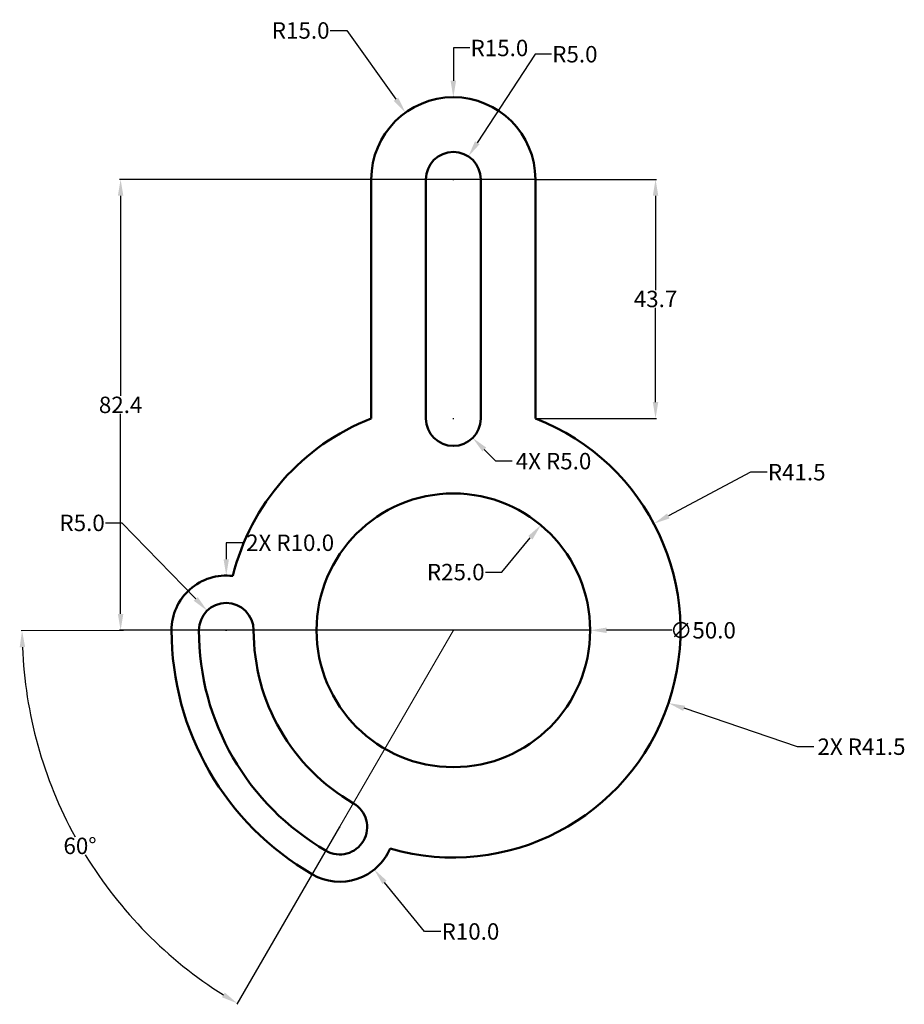
# Model space of a CAD drawing. Units: millimetres. Extents: x 927 to 1089, y 1498 to 1678.
import ezdxf

# ---------------------------------------------------------------- set-up
doc = ezdxf.new("R2010")
doc.units = ezdxf.units.MM
for name, color, linetype, lineweight in [('M-CONS', 8, 'Continuous', 13), ('M-DIMS', 2, 'Continuous', 25), ('M-OUTL', 7, 'Continuous', 50)]:
    doc.layers.add(name, color=color, linetype=linetype, lineweight=lineweight)
doc.styles.get("Standard").update_dxf_attribs({"font": 'arial.ttf'})
doc.dimstyles.get("Standard").update_dxf_attribs({"dimtxt": 3, "dimasz": 3, "dimexe": 0.18, "dimexo": 0.0625, "dimgap": 0.09, "dimtad": 0, "dimtih": 1, "dimtoh": 1, "dimdec": 1, "dimzin": 0, "dimdsep": 46, "dimtxsty": 'Standard', "dimcen": 0.09, "dimadec": 0, "dimazin": 0, "dimtfac": 1, "dimtdec": 1, "dimtofl": 0, "dimtmove": 0, "dimatfit": 3, "dimfxl": 1, "dimtolj": 1, "dimtzin": 0, "dimarcsym": 0})

# ---------------------------------------------------------------- blocks, each defined once
blk = doc.blocks.new('*D1')
at = {"layer": 'Defpoints', "color": 0, "transparency": 16777216}
for p in [(1022.42, 1585.63), (1006.43, 1566.42)]:
    blk.add_point(p, dxfattribs=at)
at = {"layer": 'M-DIMS', "color": 0, "lineweight": -2, "transparency": 16777216}
for p, q in [((1015.29, 1577.06), (1020.5, 1583.33)), ((1012.29, 1577.06), (1015.29, 1577.06))]:
    blk.add_line(p, q, dxfattribs=at)
at = {"layer": 'M-DIMS', "color": 0, "transparency": 16777216}
blk.add_solid([(1020.12, 1583.65), (1020.89, 1583.01), (1022.42, 1585.63)], dxfattribs=at)
at = {"layer": 'M-DIMS', "color": 0, "transparency": 16777216, "insert": (1006.87, 1577.06), "char_height": 3, "attachment_point": 5}
blk.add_mtext('\\A1;R25.0', dxfattribs=at)
blk = doc.blocks.new('*D2')
at = {"layer": 'Defpoints', "color": 0, "transparency": 16777216}
for p in [(1021.43, 1648.81), (1043.38, 1648.81), (1021.43, 1605.11)]:
    blk.add_point(p, dxfattribs=at)
at = {"layer": 'M-DIMS', "color": 0, "lineweight": -2, "transparency": 16777216}
for p, q in [((1021.49, 1648.81), (1043.56, 1648.81)), ((1043.38, 1645.81), (1043.38, 1628.58)), ((1043.38, 1608.11), (1043.38, 1625.34)), ((1021.49, 1605.11), (1043.56, 1605.11))]:
    blk.add_line(p, q, dxfattribs=at)
at = {"layer": 'M-DIMS', "color": 0, "transparency": 16777216}
for points in [[(1042.88, 1645.81), (1043.88, 1645.81), (1043.38, 1648.81)], [(1042.88, 1608.11), (1043.88, 1608.11), (1043.38, 1605.11)]]:
    blk.add_solid(points, dxfattribs=at)
at = {"layer": 'M-DIMS', "color": 0, "transparency": 16777216, "insert": (1043.38, 1626.96), "char_height": 3, "attachment_point": 5}
blk.add_mtext('\\A1;43.7', dxfattribs=at)
blk = doc.blocks.new('*D3')
at = {"layer": 'Defpoints', "color": 0, "transparency": 16777216}
for p in [(1043.07, 1585.9), (1006.43, 1566.42)]:
    blk.add_point(p, dxfattribs=at)
at = {"layer": 'M-DIMS', "color": 0, "lineweight": -2, "transparency": 16777216}
for p, q in [((1060.75, 1595.31), (1045.72, 1587.31)), ((1063.75, 1595.31), (1060.75, 1595.31)), ((1006.34, 1566.42), (1006.52, 1566.42)), ((1006.43, 1566.33), (1006.43, 1566.51))]:
    blk.add_line(p, q, dxfattribs=at)
at = {"layer": 'M-DIMS', "color": 0, "transparency": 16777216}
blk.add_solid([(1045.48, 1587.75), (1045.95, 1586.87), (1043.07, 1585.9)], dxfattribs=at)
at = {"layer": 'M-DIMS', "color": 0, "transparency": 16777216, "insert": (1069.18, 1595.31), "char_height": 3, "attachment_point": 5}
blk.add_mtext('\\A1;R41.5', dxfattribs=at)
blk = doc.blocks.new('*D4')
at = {"layer": 'Defpoints', "color": 0, "transparency": 16777216}
for p in [(961.45, 1570), (964.93, 1566.42)]:
    blk.add_point(p, dxfattribs=at)
at = {"layer": 'M-DIMS', "color": 0, "lineweight": -2, "transparency": 16777216}
for p, q in [((942.84, 1586.05), (945.84, 1586.05)), ((945.84, 1586.05), (959.35, 1572.15)), ((964.84, 1566.42), (965.02, 1566.42)), ((964.93, 1566.33), (964.93, 1566.51))]:
    blk.add_line(p, q, dxfattribs=at)
at = {"layer": 'M-DIMS', "color": 0, "transparency": 16777216}
blk.add_solid([(959.71, 1572.5), (959, 1571.81), (961.45, 1570)], dxfattribs=at)
at = {"layer": 'M-DIMS', "color": 0, "transparency": 16777216, "insert": (938.59, 1586.05), "char_height": 3, "attachment_point": 5}
blk.add_mtext('\\A1;R5.0', dxfattribs=at)
blk = doc.blocks.new('*D5')
at = {"layer": 'Defpoints', "color": 0, "transparency": 16777216}
for p in [(997.69, 1661), (1006.43, 1648.81)]:
    blk.add_point(p, dxfattribs=at)
at = {"layer": 'M-DIMS', "color": 0, "lineweight": -2, "transparency": 16777216}
for p, q in [((983.94, 1676.01), (986.94, 1676.01)), ((986.94, 1676.01), (995.95, 1663.44)), ((1006.34, 1648.81), (1006.52, 1648.81)), ((1006.43, 1648.72), (1006.43, 1648.9))]:
    blk.add_line(p, q, dxfattribs=at)
at = {"layer": 'M-DIMS', "color": 0, "transparency": 16777216}
blk.add_solid([(996.35, 1663.73), (995.54, 1663.15), (997.69, 1661)], dxfattribs=at)
at = {"layer": 'M-DIMS', "color": 0, "transparency": 16777216, "insert": (978.53, 1676.01), "char_height": 3, "attachment_point": 5}
blk.add_mtext('\\A1;R15.0', dxfattribs=at)
blk = doc.blocks.new('*D6')
at = {"layer": 'Defpoints', "color": 0, "transparency": 16777216}
for p in [(1009.17, 1653), (1006.43, 1648.81)]:
    blk.add_point(p, dxfattribs=at)
at = {"layer": 'M-DIMS', "color": 0, "lineweight": -2, "transparency": 16777216}
for p, q in [((1021.39, 1671.67), (1010.81, 1655.51)), ((1024.39, 1671.67), (1021.39, 1671.67)), ((1006.34, 1648.81), (1006.52, 1648.81)), ((1006.43, 1648.72), (1006.43, 1648.9))]:
    blk.add_line(p, q, dxfattribs=at)
at = {"layer": 'M-DIMS', "color": 0, "transparency": 16777216}
blk.add_solid([(1010.39, 1655.78), (1011.23, 1655.23), (1009.17, 1653)], dxfattribs=at)
at = {"layer": 'M-DIMS', "color": 0, "transparency": 16777216, "insert": (1028.64, 1671.67), "char_height": 3, "attachment_point": 5}
blk.add_mtext('\\A1;R5.0', dxfattribs=at)
blk = doc.blocks.new('*D7')
at = {"layer": 'Defpoints', "color": 0, "transparency": 16777216}
for p in [(985.68, 1530.48), (991.98, 1522.71)]:
    blk.add_point(p, dxfattribs=at)
at = {"layer": 'M-DIMS', "color": 0, "lineweight": -2, "transparency": 16777216}
for p, q in [((985.59, 1530.48), (985.77, 1530.48)), ((985.68, 1530.39), (985.68, 1530.57)), ((1001.14, 1511.4), (993.86, 1520.38)), ((1004.14, 1511.4), (1001.14, 1511.4))]:
    blk.add_line(p, q, dxfattribs=at)
at = {"layer": 'M-DIMS', "color": 0, "transparency": 16777216}
blk.add_solid([(994.25, 1520.69), (993.48, 1520.06), (991.98, 1522.71)], dxfattribs=at)
at = {"layer": 'M-DIMS', "color": 0, "transparency": 16777216, "insert": (1009.56, 1511.4), "char_height": 3, "attachment_point": 5}
blk.add_mtext('\\A1;R10.0', dxfattribs=at)
blk = doc.blocks.new('*D8')
at = {"layer": 'Defpoints', "color": 0, "transparency": 16777216}
for p in [(964.93, 1566.42), (1006.43, 1566.51), (1006.43, 1566.42), (932.4, 1539.45), (985.68, 1530.57)]:
    blk.add_point(p, dxfattribs=at)
at = {"layer": 'M-DIMS', "color": 0, "lineweight": -2, "transparency": 16777216}
for p, q in [((964.87, 1566.42), (927.44, 1566.34)), ((985.65, 1530.51), (966.89, 1498.1))]:
    blk.add_line(p, q, dxfattribs=at)
for start, end in [(182.3039, 208.6792), (211.4015, 237.7581)]:
    blk.add_arc((1006.48, 1566.51), 78.86, start, end, dxfattribs=at)
at = {"layer": 'M-DIMS', "color": 0, "transparency": 16777216}
for points in [[(927.18, 1563.33), (928.18, 1563.35), (927.62, 1566.34)], [(964.67, 1500.23), (964.15, 1499.38), (966.98, 1498.25)]]:
    blk.add_solid(points, dxfattribs=at)
at = {"layer": 'M-DIMS', "color": 0, "transparency": 16777216, "insert": (938.21, 1527.04), "char_height": 3, "attachment_point": 5}
blk.add_mtext('\\A1;60°', dxfattribs=at)
blk = doc.blocks.new('*D9')
at = {"layer": 'Defpoints', "color": 0, "transparency": 16777216}
for p in [(945.63, 1648.81), (1021.43, 1648.81), (1031.43, 1566.42)]:
    blk.add_point(p, dxfattribs=at)
at = {"layer": 'M-DIMS', "color": 0, "lineweight": -2, "transparency": 16777216}
for p, q in [((1021.37, 1648.81), (945.45, 1648.81)), ((945.63, 1645.81), (945.63, 1609.24)), ((945.63, 1569.42), (945.63, 1605.99)), ((1031.37, 1566.42), (945.45, 1566.42))]:
    blk.add_line(p, q, dxfattribs=at)
at = {"layer": 'M-DIMS', "color": 0, "transparency": 16777216}
for points in [[(945.13, 1645.81), (946.13, 1645.81), (945.63, 1648.81)], [(945.13, 1569.42), (946.13, 1569.42), (945.63, 1566.42)]]:
    blk.add_solid(points, dxfattribs=at)
at = {"layer": 'M-DIMS', "color": 0, "transparency": 16777216, "insert": (945.63, 1607.61), "char_height": 3, "attachment_point": 5}
blk.add_mtext('\\A1;82.4', dxfattribs=at)
blk = doc.blocks.new('*D10')
at = {"layer": 'Defpoints', "color": 0, "transparency": 16777216}
for p in [(981.43, 1566.42), (1031.43, 1566.42)]:
    blk.add_point(p, dxfattribs=at)
at = {"layer": 'M-DIMS', "color": 0, "lineweight": -2, "transparency": 16777216}
for p, q in [((1006.34, 1566.42), (1006.52, 1566.42)), ((1006.43, 1566.33), (1006.43, 1566.51)), ((1046.43, 1566.42), (1034.43, 1566.42))]:
    blk.add_line(p, q, dxfattribs=at)
at = {"layer": 'M-DIMS', "color": 0, "transparency": 16777216}
blk.add_solid([(1034.43, 1566.92), (1034.43, 1565.92), (1031.43, 1566.42)], dxfattribs=at)
at = {"layer": 'M-DIMS', "color": 0, "transparency": 16777216, "insert": (1052.04, 1566.42), "char_height": 3, "attachment_point": 5}
blk.add_mtext('\\A1;∅50.0', dxfattribs=at)
blk = doc.blocks.new('*D11')
at = {"layer": 'Defpoints', "color": 0, "transparency": 16777216}
for p in [(1006.43, 1566.42), (1045.75, 1553.13)]:
    blk.add_point(p, dxfattribs=at)
at = {"layer": 'M-DIMS', "color": 0, "lineweight": -2, "transparency": 16777216}
for p, q in [((1006.34, 1566.42), (1006.52, 1566.42)), ((1006.43, 1566.33), (1006.43, 1566.51)), ((1069.33, 1545.16), (1048.59, 1552.17)), ((1072.33, 1545.16), (1069.33, 1545.16))]:
    blk.add_line(p, q, dxfattribs=at)
at = {"layer": 'M-DIMS', "color": 0, "transparency": 16777216}
blk.add_solid([(1048.75, 1552.64), (1048.43, 1551.69), (1045.75, 1553.13)], dxfattribs=at)
at = {"layer": 'M-DIMS', "color": 0, "transparency": 16777216, "insert": (1081.02, 1545.16), "char_height": 3, "attachment_point": 5}
blk.add_mtext('\\A1;2X R41.5', dxfattribs=at)
blk = doc.blocks.new('*D12')
at = {"layer": 'Defpoints', "color": 0, "transparency": 16777216}
for p in [(1006.43, 1663.81), (1006.43, 1648.81)]:
    blk.add_point(p, dxfattribs=at)
at = {"layer": 'M-DIMS', "color": 0, "lineweight": -2, "transparency": 16777216}
for p, q in [((1009.43, 1672.81), (1006.43, 1672.81)), ((1006.43, 1672.81), (1006.43, 1666.81)), ((1006.34, 1648.81), (1006.52, 1648.81)), ((1006.43, 1648.72), (1006.43, 1648.9))]:
    blk.add_line(p, q, dxfattribs=at)
at = {"layer": 'M-DIMS', "color": 0, "transparency": 16777216}
blk.add_solid([(1005.93, 1666.81), (1006.93, 1666.81), (1006.43, 1663.81)], dxfattribs=at)
at = {"layer": 'M-DIMS', "color": 0, "transparency": 16777216, "insert": (1014.85, 1672.81), "char_height": 3, "attachment_point": 5}
blk.add_mtext('\\A1;R15.0', dxfattribs=at)
blk = doc.blocks.new('*D13')
at = {"layer": 'Defpoints', "color": 0, "transparency": 16777216}
for p in [(1006.43, 1605.11), (1009.97, 1601.57)]:
    blk.add_point(p, dxfattribs=at)
at = {"layer": 'M-DIMS', "color": 0, "lineweight": -2, "transparency": 16777216}
for p, q in [((1006.34, 1605.11), (1006.52, 1605.11)), ((1006.43, 1605.02), (1006.43, 1605.2)), ((1014.21, 1597.33), (1012.09, 1599.45)), ((1017.21, 1597.33), (1014.21, 1597.33))]:
    blk.add_line(p, q, dxfattribs=at)
at = {"layer": 'M-DIMS', "color": 0, "transparency": 16777216}
blk.add_solid([(1012.44, 1599.81), (1011.73, 1599.1), (1009.97, 1601.57)], dxfattribs=at)
at = {"layer": 'M-DIMS', "color": 0, "transparency": 16777216, "insert": (1024.74, 1597.33), "char_height": 3, "attachment_point": 5}
blk.add_mtext('\\A1;4X R5.0', dxfattribs=at)
blk = doc.blocks.new('*D14')
at = {"layer": 'Defpoints', "color": 0, "transparency": 16777216}
for p in [(964.93, 1576.42), (964.93, 1566.42)]:
    blk.add_point(p, dxfattribs=at)
at = {"layer": 'M-DIMS', "color": 0, "lineweight": -2, "transparency": 16777216}
for p, q in [((967.93, 1582.42), (964.93, 1582.42)), ((964.93, 1582.42), (964.93, 1579.42)), ((964.84, 1566.42), (965.02, 1566.42)), ((964.93, 1566.33), (964.93, 1566.51))]:
    blk.add_line(p, q, dxfattribs=at)
at = {"layer": 'M-DIMS', "color": 0, "transparency": 16777216}
blk.add_solid([(964.43, 1579.42), (965.43, 1579.42), (964.93, 1576.42)], dxfattribs=at)
at = {"layer": 'M-DIMS', "color": 0, "transparency": 16777216, "insert": (976.6, 1582.42), "char_height": 3, "attachment_point": 5}
blk.add_mtext('\\A1;2X R10.0', dxfattribs=at)

msp = doc.modelspace()

# ---------------------------------------------------------------- linework, layer by layer
at = {"layer": 'M-CONS'}
for p, q in [((1001.43, 1590.97), (1001.43, 1590.91)), ((1011.43, 1590.97), (1011.43, 1590.91)), ((964.93, 1566.42), (1006.43, 1566.51)), ((1006.34, 1566.42), (969.93, 1566.42)), ((1006.43, 1566.42), (985.68, 1530.57))]:
    msp.add_line(p, q, dxfattribs=at)
for start, end in [(250.5288, 250.9492), (289.0508, 289.4712)]:
    msp.add_arc((1006.43, 1605.11), 15, start, end, dxfattribs=at)
at = {"layer": 'M-OUTL'}
for p, q in [((991.43, 1605.11), (991.43, 1648.81)), ((1001.43, 1648.81), (1001.43, 1605.11)), ((1011.43, 1648.81), (1011.43, 1605.11)), ((1021.43, 1605.11), (1021.43, 1648.81)), ((1021.43, 1605.11), (1021.43, 1648.81))]:
    msp.add_line(p, q, dxfattribs=at)
msp.add_circle((1006.43, 1566.42), 25, dxfattribs=at)
for centre, radius, start, end in [((1006.43, 1648.81), 15, 0, 180), ((1006.43, 1648.81), 5, 0, 180), ((1006.43, 1566.42), 41.5, 111.189, 166.1602), ((1006.43, 1566.42), 41.5, 253.8398, 68.811), ((1006.43, 1605.11), 5, 180, 0), ((964.93, 1566.42), 10, 83.0801, 180), ((964.93, 1566.42), 5, 0, 180), ((1006.43, 1566.42), 51.5, 180, 240), ((1006.43, 1566.42), 46.5, 180, 240), ((1006.43, 1566.42), 36.5, 180, 240), ((985.68, 1530.48), 5, 240, 60), ((985.68, 1530.48), 10, 240, 336.9199)]:
    msp.add_arc(centre, radius, start, end, dxfattribs=at)

# ---------------------------------------------------------------- dimensions: what is measured, and where the dimension line sits
at = {"layer": 'M-DIMS'}
for center, mpoint, override, picture, middle in [((1006.43, 1648.81), (997.69, 1661), {"dimclrd": 0, "dimclre": 0, "dimclrt": 0}, '*D5', (978.53, 1676.01)), ((1006.43, 1648.81), (1006.43, 1663.81), {"dimdec": 1, "dimlfac": 1, "dimrnd": 0, "dimzin": 0, "dimdsep": 46, "dimlunit": 2}, '*D12', (1014.85, 1672.81)), ((1006.43, 1648.81), (1009.17, 1653), {"dimclrd": 0, "dimclre": 0, "dimclrt": 0}, '*D6', (1028.64, 1671.67)), ((1006.43, 1566.42), (1043.07, 1585.9), {"dimclrd": 0, "dimclre": 0, "dimclrt": 0}, '*D3', (1069.18, 1595.31)), ((964.93, 1566.42), (961.45, 1570), {"dimclrd": 0, "dimclre": 0, "dimclrt": 0}, '*D4', (938.59, 1586.05)), ((1006.43, 1566.42), (1022.42, 1585.63), {"dimclrd": 0, "dimclre": 0, "dimclrt": 0}, '*D1', (1006.87, 1577.06)), ((985.68, 1530.48), (991.98, 1522.71), {"dimclrd": 0, "dimclre": 0, "dimclrt": 0}, '*D7', (1009.56, 1511.4))]:
    dim = msp.add_radius_dim(center=center, mpoint=mpoint, dimstyle='Standard', override=override, dxfattribs=at)
    dim.commit()
    dim.dimension.update_dxf_attribs({"geometry": picture, "text_midpoint": middle, "dimtype": 164})
for base, p1, override, picture, middle in [((945.63, 1648.81), (1031.43, 1566.42), {"dimdec": 1, "dimlfac": 1, "dimrnd": 0, "dimzin": 0, "dimdsep": 46, "dimlunit": 2}, '*D9', (945.63, 1607.61)), ((1043.38, 1648.81), (1021.43, 1605.11), {"dimclrd": 0, "dimclre": 0, "dimclrt": 0}, '*D2', (1043.38, 1626.96))]:
    dim = msp.add_linear_dim(base=base, p1=p1, p2=(1021.43, 1648.81), angle=90, dimstyle='Standard', override=override, dxfattribs=at)
    dim.commit()
    dim.dimension.update_dxf_attribs({"geometry": picture, "text_midpoint": middle})
dim = msp.add_radius_dim(center=(1006.43, 1605.11), mpoint=(1009.97, 1601.57), text='4X <>', dimstyle='Standard', override={"dimdec": 1, "dimlfac": 1, "dimrnd": 0, "dimzin": 0, "dimdsep": 46, "dimlunit": 2}, dxfattribs=at)
dim.commit()
dim.dimension.update_dxf_attribs({"geometry": '*D13', "text_midpoint": (1024.74, 1597.33)})
for center, mpoint, picture, middle in [((964.93, 1566.42), (964.93, 1576.42), '*D14', (976.6, 1582.42)), ((1006.43, 1566.42), (1045.75, 1553.13), '*D11', (1081.02, 1545.16))]:
    dim = msp.add_radius_dim(center=center, mpoint=mpoint, text='2X <>', dimstyle='Standard', override={"dimdec": 1, "dimlfac": 1, "dimrnd": 0, "dimzin": 0, "dimdsep": 46, "dimlunit": 2}, dxfattribs=at)
    dim.commit()
    dim.dimension.update_dxf_attribs({"geometry": picture, "text_midpoint": middle, "dimtype": 164})
dim = msp.add_diameter_dim_2p(p1=(981.43, 1566.42), p2=(1031.43, 1566.42), dimstyle='Standard', override={"dimdec": 1, "dimlfac": 1, "dimrnd": 0, "dimzin": 0, "dimdsep": 46, "dimlunit": 2}, dxfattribs=at)
dim.commit()
dim.dimension.update_dxf_attribs({"geometry": '*D10', "text_midpoint": (1046.43, 1566.42), "dimtype": 163})
dim = msp.add_angular_dim_2l(base=(932.4, 1539.45), line1=((964.93, 1566.42), (1006.43, 1566.51)), line2=((1006.43, 1566.42), (985.68, 1530.57)), dimstyle='Standard', override={"dimclrd": 0, "dimclre": 0, "dimclrt": 0}, dxfattribs=at)
dim.commit()
dim.dimension.update_dxf_attribs({"geometry": '*D8', "text_midpoint": (938.21, 1527.04)})

doc.saveas('drawing.dxf')
